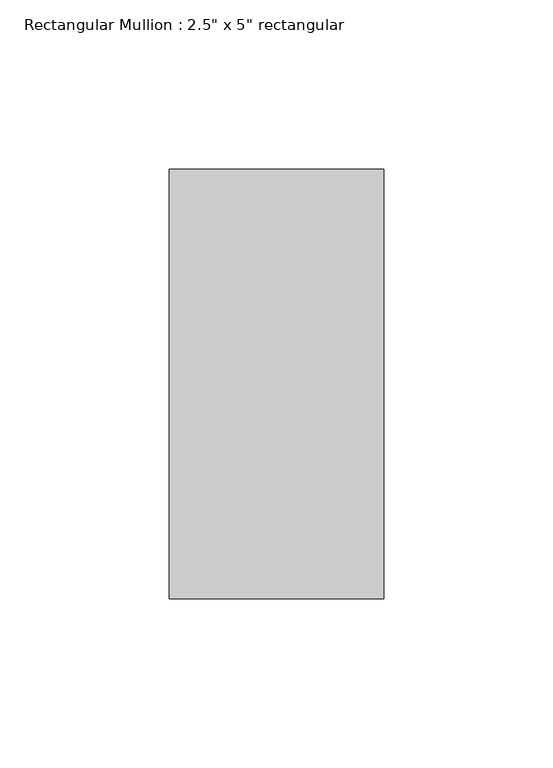
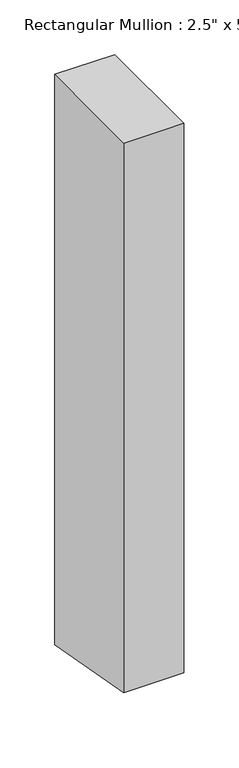
"""IFC4 building model written with IfcOpenShell, lengths in millimetres: member geometry."""

from ifc_helpers import new_model, si_unit, frame, origin, place, context, project, spatial, polyline, outline, extrude, source, transform, mapped, element, save


def member_83685764(model_context):
    return source(origin(), model_context, "Body", "SweptSolid", [
        extrude(outline(polyline([(-63.5, 0.0), (63.5, 0.0), (63.5, -637.4452824), (-63.5, -614.2374121), (-63.5, 0.0)])), frame((-63.5, 0.0, 0.0), z_axis=(1.0, 0.0, 0.0), x_axis=(0.0, 1.0, 0.0)), (0.0, 0.0, 1.0), 63.5),
    ])


if __name__ == "__main__":
    model = new_model("IFC4")
    model_context = context("Model", 3, world=origin())
    ifc_project = project(units=[si_unit("LENGTHUNIT", "METRE", prefix="MILLI")], contexts=[model_context])
    site = spatial("IfcSite", under=ifc_project)
    building = spatial("IfcBuilding", under=site)
    placement = place(None, origin())
    member_shape = member_83685764(model_context)
    element("IfcMember", 1, ObjectType="Rectangular Mullion : 2.5\" x 5\" rectangular", at=placement, inside=building, context=model_context, shape_type="MappedRepresentation", body=[
        mapped(member_shape, transform((0.0, 0.0, 0.0), x_axis=(1.0, 0.0, 0.0), y_axis=(0.0, 1.0, 0.0), z_axis=(0.0, 0.0, 1.0))),
    ])
    save(model, "model.ifc")

# Revit data of these elements
# Type "Rectangular Mullion : 2.5\" x 5\" rectangular"
#   built-in parameter 1007304 = 0.416667 (stored number, unit not read)
#   built-in parameter 1007301 = 0.104167 (stored number, unit not read)
#   built-in parameter 1007300 = 0.104167 (stored number, unit not read)
# Element 1 (IfcMember, "Rectangular Mullion : 2.5\" x 5\" rectangular")
#   Materials on its faces: "Iron, Ductile"
# Materials
#   "Iron, Ductile": class "Metal", colour RGB 0 0 0, transparency 0, Description = "Ductile cast iron", Cost = 0
